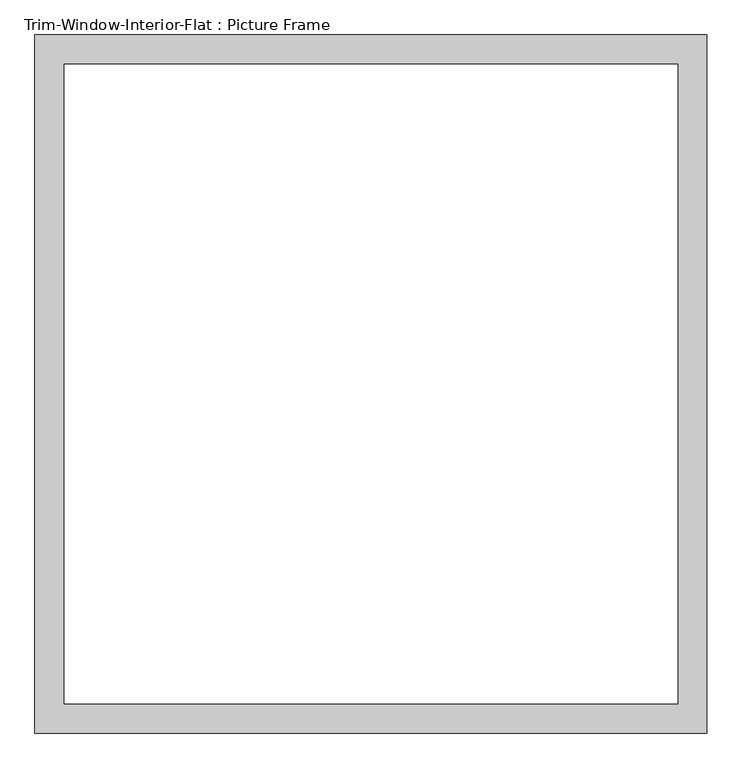
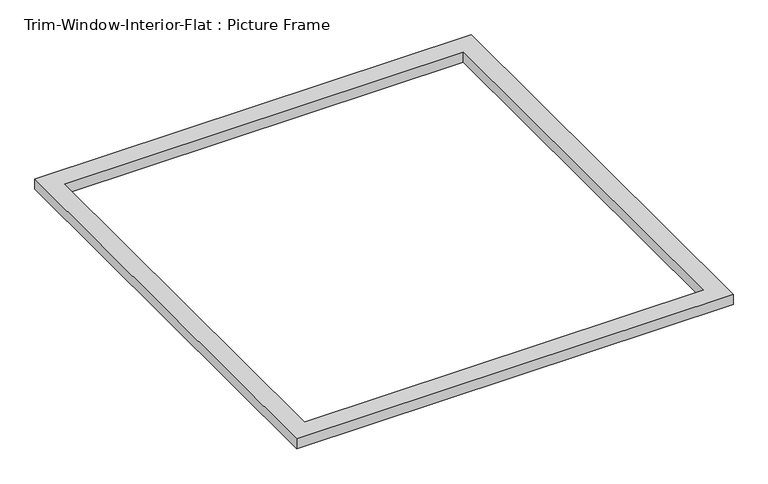
"""IFC4 building model written with IfcOpenShell, lengths in millimetres: proxy geometry, Trim-Window-Interior-Flat : Picture Frame."""

from ifc_helpers import new_model, si_unit, origin, origin_with_axes, place, context, project, spatial, polyline, outline, extrude, source, transform, mapped, element, save


def trim_window_interior_flat_picture_frame_ace0ae79(model_context):
    return source(origin(), model_context, "Body", "SweptSolid", [
        extrude(outline(polyline([(654.05, 44.45), (654.05, -1314.45), (-654.05, -1314.45), (-654.05, 44.45), (654.05, 44.45)]), holes=[polyline([(596.9, -12.7), (-596.9, -12.7), (-596.9, -1257.3), (596.9, -1257.3), (596.9, -12.7)])]), origin_with_axes(), (0.0, 0.0, 1.0), 31.75),
    ])


if __name__ == "__main__":
    model = new_model("IFC4")
    model_context = context("Model", 3, world=origin())
    ifc_project = project(units=[si_unit("LENGTHUNIT", "METRE", prefix="MILLI")], contexts=[model_context])
    site = spatial("IfcSite", under=ifc_project)
    building = spatial("IfcBuilding", under=site)
    placement = place(None, origin())
    trim_window_interior_flat_picture_frame_shape = trim_window_interior_flat_picture_frame_ace0ae79(model_context)
    element("IfcBuildingElementProxy", 1, Name="Trim-Window-Interior-Flat : Picture Frame", ObjectType="Trim-Window-Interior-Flat : Picture Frame", at=placement, inside=building, context=model_context, shape_type="MappedRepresentation", body=[
        mapped(trim_window_interior_flat_picture_frame_shape, transform((0.0, 0.0, 0.0), x_axis=(1.0, 0.0, 0.0), y_axis=(0.0, 1.0, 0.0), z_axis=(0.0, 0.0, 1.0))),
    ])
    save(model, "model.ifc")

# Revit data of these elements
# Type "Trim-Window-Interior-Flat : Picture Frame"
#   Trim Thickness_Picture Frame = 0' - 1 1/4"
#   Trim Width = 0' - 2 1/4"
#   Trim Thickness_with Sill = 0' - 0 3/4"
#   Sill Thickness = 0' - 1 1/4"
#   Opening Width [instance default] = 2' - 0"
#   Opening Height [instance default] = 3' - 0"
#   Default Elevation = 4' - 0"
#   Sill = no
#   Picture Frame = yes
#   Trim Material [instance default] = none
# Element 1 (IfcBuildingElementProxy, "Trim-Window-Interior-Flat : Picture Frame")
#   Opening Width = 4' - 0"
#   Opening Height = 4' - 2"
#   Trim Material = Wood - Stained
#   Materials on its faces: "Wood - Stained"
# Materials
#   "Wood - Stained": class "Wood", colour RGB 224 178 126, transparency 0, Cost = 0
